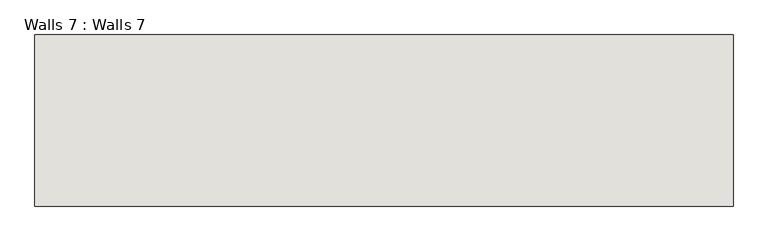
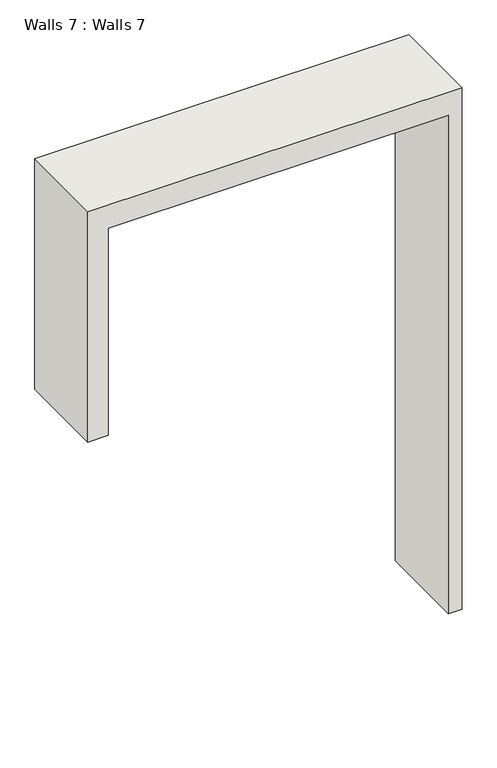
"""IFC4 building model written with IfcOpenShell, lengths in millimetres: wall geometry, Walls 7 : Walls 7."""

from ifc_helpers import new_model, si_unit, frame, origin, place, context, project, spatial, polyline, outline, extrude, source, transform, mapped, element, save


def walls_7_walls_7_eccbc88b(model_context):
    return source(origin(), model_context, "Body", "SweptSolid", [
        extrude(outline(polyline([(3048.0, -6306.4066261), (3048.0, -6171.9407032), (8510.6708804, -6171.9407032), (8510.6708804, -9880.3407032), (6096.0, -9880.3407032), (6096.0, -9680.3407032), (8267.2163813, -9680.3407032), (8267.2163813, -6306.4066261), (3048.0, -6306.4066261)])), frame((0.0, 3251.3956099, 0.0), z_axis=(0.0, 1.0, 0.0), x_axis=(0.0, 0.0, 1.0)), (0.0, 0.0, 1.0), 911.0079546),
    ])


if __name__ == "__main__":
    model = new_model("IFC4")
    model_context = context("Model", 3, world=origin())
    ifc_project = project(units=[si_unit("LENGTHUNIT", "METRE", prefix="MILLI")], contexts=[model_context])
    site = spatial("IfcSite", under=ifc_project)
    building = spatial("IfcBuilding", under=site)
    placement = place(None, origin())
    walls_7_walls_7_shape = walls_7_walls_7_eccbc88b(model_context)
    element("IfcWall", 1, ObjectType="Walls 7 : Walls 7", at=placement, inside=building, context=model_context, shape_type="MappedRepresentation", body=[
        mapped(walls_7_walls_7_shape, transform((0.0, 0.0, 0.0), x_axis=(1.0, 0.0, 0.0), y_axis=(0.0, 1.0, 0.0), z_axis=(0.0, 0.0, 1.0))),
    ])
    save(model, "model.ifc")

# Revit data of these elements
# Element 1 (IfcWall, "Walls 7 : Walls 7")
#   Materials on its faces: "Default Wall"
# Materials
#   "Default Wall": colour RGB 80 80 80, transparency 0
